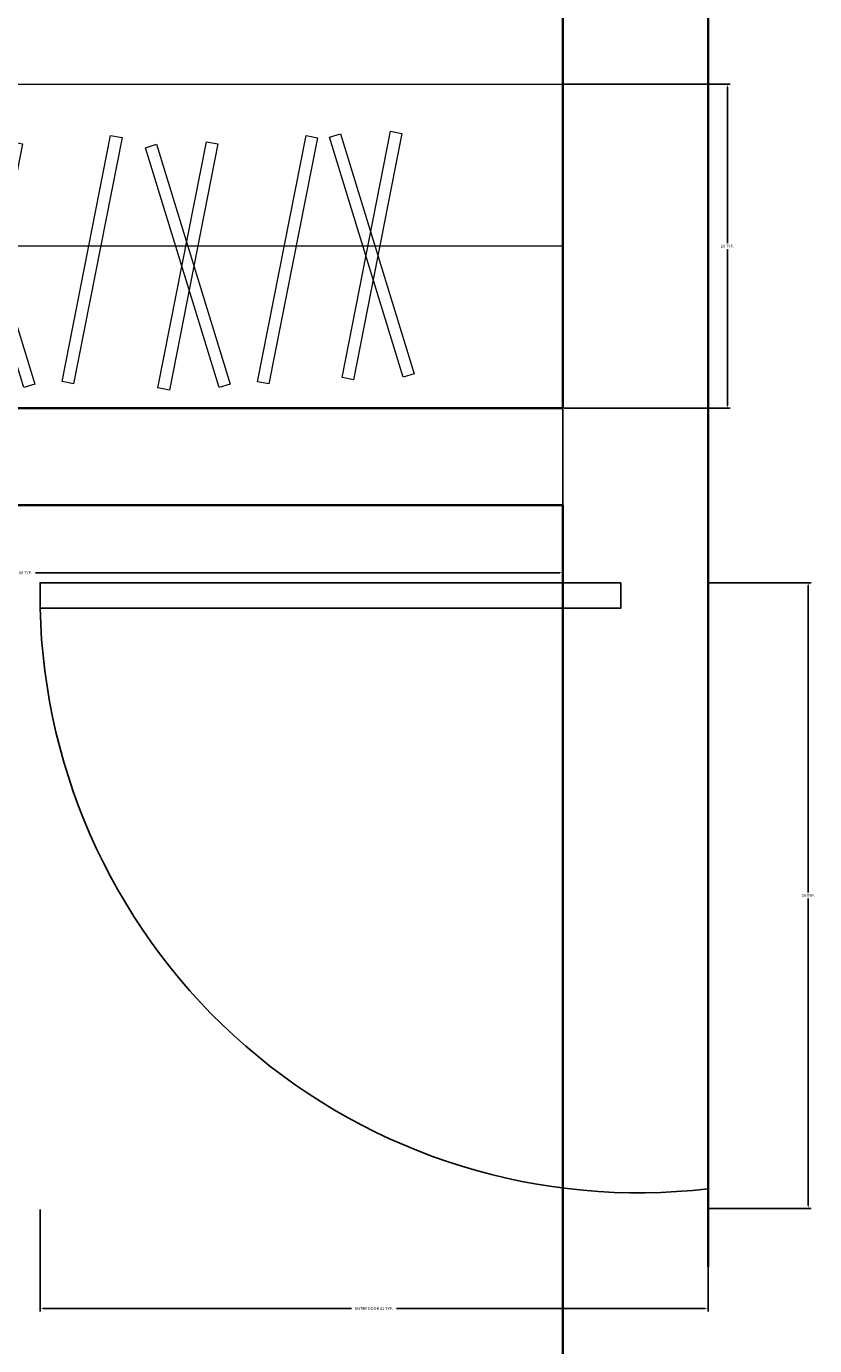
# Model space of a CAD drawing. Units: inches. Extents: x -61 to 1599, y -1316 to 257.
# Tile 181 of 204: x 1480 to 1529, y -835 to -753. Entities that reach past the tile are written whole.
import ezdxf

# ---------------------------------------------------------------- set-up
doc = ezdxf.new("R2010")
doc.units = ezdxf.units.IN
doc.header["$MEASUREMENT"] = 0
for name, color, linetype, lineweight in [('A-ANNO-DIMS', 2, 'Continuous', 18), ('A-FLOR-CASE', 8, 'Continuous', 18), ('DOORS', 2, 'Continuous', 25), ('WALLS', 4, 'Continuous', 35)]:
    doc.layers.add(name, color=color, linetype=linetype, lineweight=lineweight)
doc.styles.get("Standard").update_dxf_attribs({"font": 'arial.ttf'})
doc.dimstyles.get("Standard").update_dxf_attribs({"dimtxt": 0.18, "dimasz": 0.18, "dimexe": 0.18, "dimexo": 0.0625, "dimgap": 0.09, "dimtad": 0, "dimtih": 1, "dimtoh": 1, "dimdec": 0, "dimzin": 0, "dimdsep": 46, "dimlunit": 3, "dimtxsty": 'Standard', "dimcen": 0.09, "dimadec": 0, "dimazin": 0, "dimtfac": 1, "dimtdec": 0, "dimtofl": 0, "dimtmove": 0, "dimatfit": 3, "dimfxl": 1, "dimtolj": 1, "dimtzin": 0, "dimarcsym": 0})

# ---------------------------------------------------------------- blocks, each defined once
blk = doc.blocks.new('DOOR-SWING-36-ALT')
blk.add_lwpolyline([(0, 0), (-36, 0), (-36, -1.575), (0, -1.575)], close=True)
blk.add_arc((1.079, -0.739), 37.088, 181.2913, 276.69053)
blk = doc.blocks.new('WARDROBE-HANGING-4')
blk.add_line((68, 10.047), (0, 10.047))
for points in [[(68, 20.094), (68, 0), (0, 0), (0, 20.094)], [(0.148, 2.482), (3.151, 17.75), (3.858, 17.611), (0.854, 2.343)], [(8.838, 1.346), (4.269, 16.221), (4.957, 16.432), (9.526, 1.557)], [(5.043, 1.324), (8.046, 16.593), (8.753, 16.454), (5.749, 1.185)], [(11.216, 1.713), (14.219, 16.981), (14.925, 16.842), (11.922, 1.574)], [(17.985, 1.394), (20.989, 16.662), (21.695, 16.523), (18.692, 1.255)], [(23.91, 1.364), (26.914, 16.633), (27.62, 16.494), (24.617, 1.225)], [(34.592, 1.283), (30.023, 16.158), (30.711, 16.37), (35.28, 1.495)], [(30.797, 1.262), (33.8, 16.53), (34.507, 16.391), (31.503, 1.123)], [(36.97, 1.651), (39.973, 16.919), (40.68, 16.78), (37.676, 1.512)], [(46.701, 1.279), (42.132, 16.153), (42.82, 16.365), (47.389, 1.49)], [(42.906, 1.257), (45.909, 16.525), (46.616, 16.386), (43.612, 1.118)], [(49.079, 1.646), (52.082, 16.914), (52.788, 16.775), (49.785, 1.507)], [(58.108, 1.928), (53.539, 16.802), (54.227, 17.014), (58.796, 2.139)], [(54.313, 1.906), (57.316, 17.174), (58.023, 17.035), (55.019, 1.767)], [(21.533, 0.997), (16.964, 15.872), (17.652, 16.083), (22.221, 1.209)]]:
    blk.add_lwpolyline(points, close=True)
blk = doc.blocks.new('*D678')
at = {"layer": 'A-ANNO-DIMS', "color": 0, "lineweight": -2, "transparency": 16777216}
for p, q in [((1481.303, -826.842), (1481.303, -833.17)), ((1522.703, -826.842), (1522.703, -833.17)), ((1481.483, -832.99), (1500.606, -832.99)), ((1522.523, -832.99), (1503.399, -832.99))]:
    blk.add_line(p, q, dxfattribs=at)
at = {"layer": 'A-ANNO-DIMS', "color": 0, "transparency": 16777216}
for points in [[(1481.483, -832.96), (1481.483, -833.02), (1481.303, -832.99)], [(1522.523, -832.96), (1522.523, -833.02), (1522.703, -832.99)]]:
    blk.add_solid(points, dxfattribs=at)
at = {"layer": 'DEFPOINTS', "color": 0, "transparency": 16777216}
for p in [(1481.303, -826.78), (1522.703, -826.78), (1522.703, -832.99)]:
    blk.add_point(p, dxfattribs=at)
at = {"layer": 'A-ANNO-DIMS', "color": 0, "transparency": 16777216, "insert": (1502.003, -832.99), "char_height": 0.18, "attachment_point": 5}
blk.add_mtext('\\A1;ENTRY DOOR 41 TYP.', dxfattribs=at)
blk = doc.blocks.new('*D679')
at = {"layer": 'A-ANNO-DIMS', "color": 0, "lineweight": -2, "transparency": 16777216}
for p, q in [((1522.765, -787.988), (1529.093, -787.988)), ((1528.913, -788.168), (1528.913, -807.202)), ((1528.913, -826.6), (1528.913, -807.566)), ((1522.765, -826.78), (1529.093, -826.78))]:
    blk.add_line(p, q, dxfattribs=at)
at = {"layer": 'A-ANNO-DIMS', "color": 0, "transparency": 16777216}
for points in [[(1528.883, -788.168), (1528.943, -788.168), (1528.913, -787.988)], [(1528.883, -826.6), (1528.943, -826.6), (1528.913, -826.78)]]:
    blk.add_solid(points, dxfattribs=at)
at = {"layer": 'DEFPOINTS', "color": 0, "transparency": 16777216}
for p in [(1522.703, -787.988), (1528.913, -787.988), (1522.703, -826.78)]:
    blk.add_point(p, dxfattribs=at)
at = {"layer": 'A-ANNO-DIMS', "color": 0, "transparency": 16777216, "insert": (1528.913, -807.384), "char_height": 0.18, "attachment_point": 5}
blk.add_mtext('\\A1;39 TYP.', dxfattribs=at)
blk = doc.blocks.new('*D680')
at = {"layer": 'A-ANNO-DIMS', "color": 0, "lineweight": -2, "transparency": 16777216}
for p, q in [((1445.703, -777.232), (1445.703, -787.549)), ((1513.703, -777.232), (1513.703, -787.549)), ((1445.883, -787.369), (1478.396, -787.369)), ((1513.523, -787.369), (1481.01, -787.369))]:
    blk.add_line(p, q, dxfattribs=at)
at = {"layer": 'A-ANNO-DIMS', "color": 0, "transparency": 16777216}
for points in [[(1445.883, -787.339), (1445.883, -787.399), (1445.703, -787.369)], [(1513.523, -787.339), (1513.523, -787.399), (1513.703, -787.369)]]:
    blk.add_solid(points, dxfattribs=at)
at = {"layer": 'DEFPOINTS', "color": 0, "transparency": 16777216}
for p in [(1445.703, -777.169), (1513.703, -777.169), (1513.703, -787.369)]:
    blk.add_point(p, dxfattribs=at)
at = {"layer": 'A-ANNO-DIMS', "color": 0, "transparency": 16777216, "insert": (1479.703, -787.369), "char_height": 0.18, "attachment_point": 5}
blk.add_mtext('\\A1;WARDROBE 68 TYP.', dxfattribs=at)
blk = doc.blocks.new('*D681')
at = {"layer": 'A-ANNO-DIMS', "color": 0, "lineweight": -2, "transparency": 16777216}
for p, q in [((1513.765, -757.075), (1524.083, -757.075)), ((1523.903, -757.255), (1523.903, -766.94)), ((1523.903, -776.989), (1523.903, -767.304)), ((1513.765, -777.169), (1524.083, -777.169))]:
    blk.add_line(p, q, dxfattribs=at)
at = {"layer": 'A-ANNO-DIMS', "color": 0, "transparency": 16777216}
for points in [[(1523.873, -757.255), (1523.933, -757.255), (1523.903, -757.075)], [(1523.873, -776.989), (1523.933, -776.989), (1523.903, -777.169)]]:
    blk.add_solid(points, dxfattribs=at)
at = {"layer": 'DEFPOINTS', "color": 0, "transparency": 16777216}
for p in [(1513.703, -757.075), (1523.903, -757.075), (1513.703, -777.169)]:
    blk.add_point(p, dxfattribs=at)
at = {"layer": 'A-ANNO-DIMS', "color": 0, "transparency": 16777216, "insert": (1523.903, -767.122), "char_height": 0.18, "attachment_point": 5}
blk.add_mtext('\\A1;20 TYP.', dxfattribs=at)

msp = doc.modelspace()

# ---------------------------------------------------------------- linework, layer by layer
at = {"layer": 'WALLS'}
for p, q in [((1513.7028, -621.169), (1513.7028, -777.169)), ((1522.7028, -830.3954), (1522.7028, -735.0151)), ((1375.7028, -777.169), (1513.7028, -777.169)), ((1375.7028, -783.169), (1513.7028, -783.169)), ((1513.7028, -783.169), (1513.7028, -945.169))]:
    msp.add_line(p, q, dxfattribs=at)

# ---------------------------------------------------------------- block references
at = {"layer": 'A-FLOR-CASE'}
msp.add_blockref('WARDROBE-HANGING-4', (1445.703, -777.1691), dxfattribs=at)
at = {"layer": 'DOORS'}
msp.add_blockref('DOOR-SWING-36-ALT', (1517.3028, -787.9879), dxfattribs=at)

# ---------------------------------------------------------------- dimensions: what is measured, and where the dimension line sits
at = {"layer": 'A-ANNO-DIMS'}
for base, p1, p2, picture, middle in [((1523.9028, -757.0754), (1513.7028, -777.169), (1513.7028, -757.0754), '*D681', (1523.9028, -767.1222)), ((1528.9128, -787.9879), (1522.7028, -826.7796), (1522.7028, -787.9879), '*D679', (1528.9128, -807.3838))]:
    dim = msp.add_linear_dim(base=base, p1=p1, p2=p2, angle=90, text='<> TYP.', dimstyle='Standard', override={"dimdec": 0, "dimlfac": 1, "dimrnd": 0, "dimzin": 0, "dimdsep": 46, "dimlunit": 2}, dxfattribs=at)
    dim.commit()
    dim.dimension.update_dxf_attribs({"geometry": picture, "text_midpoint": middle})
for base, p1, p2, text, picture, middle in [((1513.7028, -787.369), (1445.7028, -777.169), (1513.7028, -777.169), 'WARDROBE <> TYP.', '*D680', (1479.7028, -787.369)), ((1522.7028, -832.9896), (1481.3028, -826.7796), (1522.7028, -826.7796), 'ENTRY DOOR <> TYP.', '*D678', (1502.0028, -832.9896))]:
    dim = msp.add_linear_dim(base=base, p1=p1, p2=p2, text=text, dimstyle='Standard', override={"dimdec": 0, "dimlfac": 1, "dimrnd": 0, "dimzin": 0, "dimdsep": 46, "dimlunit": 2}, dxfattribs=at)
    dim.commit()
    dim.dimension.update_dxf_attribs({"geometry": picture, "text_midpoint": middle})

doc.saveas('drawing.dxf')
